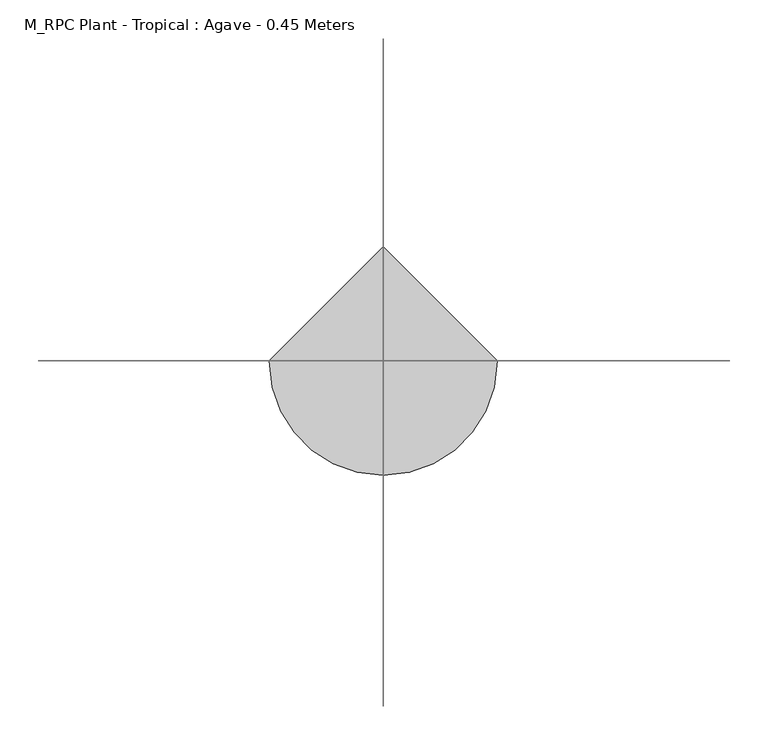
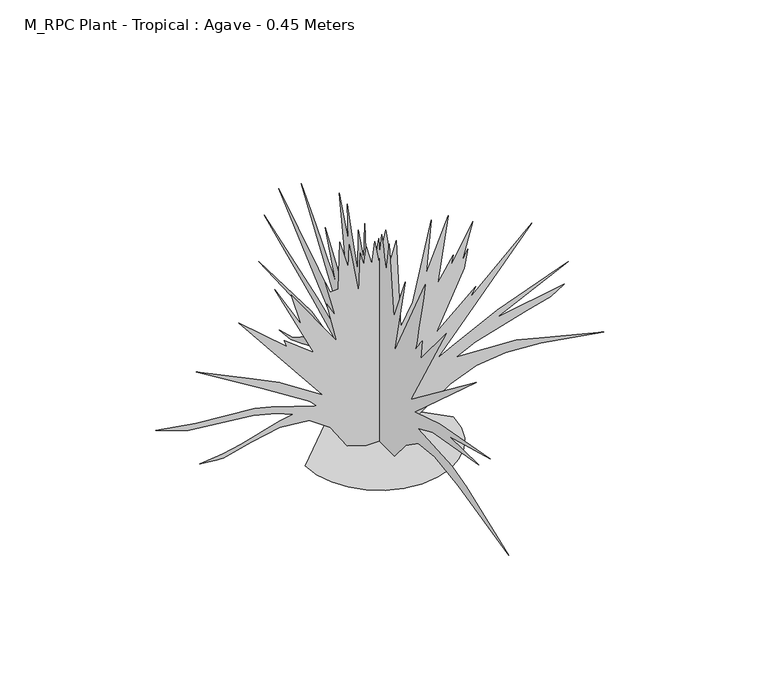
"""IFC4 building model written with IfcOpenShell, lengths in millimetres: geographic element geometry, M_RPC Plant - Tropical : Agave - 0.45 Meters."""

from ifc_helpers import new_model, si_unit, origin, place, context, project, spatial, triangles, source, transform, mapped, element, save


def m_rpc_plant_tropical_agave_0_45_meters_eb57889b(model_context):
    return source(origin(), model_context, "Body", "Tessellation", [
        triangles([(-148.1386958, 0.0, 9.3e-06), (-144.2171964, -33.9885277, 9.3e-06), (-133.048683, -65.2018023, 9.3e-06), (-115.5276685, -92.7450748, 9.3e-06), (-92.5484025, -115.7243407, 9.3e-06), (-65.0051301, -133.2453552, 9.3e-06), (-33.7918577, -144.4138686, 9.3e-06), (0.1966776, -148.335368, 9.3e-06), (34.1851976, -144.4138686, 9.3e-06), (65.3984745, -133.2453552, 9.3e-06), (92.941747, -115.7243407, 9.3e-06), (115.921013, -92.7450748, 9.3e-06), (133.4420274, -65.2018023, 9.3e-06), (144.6105409, -33.9885277, 9.3e-06), (148.5320402, 1.3e-05, 9.3e-06), (0.1966516, 148.335368, 9.3e-06), (-24.3504237, 1.1e-06, 2.5e-06), (-64.1988793, 2e-06, 12.9348607), (-97.895905, 5e-07, 64.0713026), (-140.594189, 5e-07, 94.1593235), (-198.9417449, 2.8e-06, 99.5475756), (-255.4485429, 5.9e-06, 87.7748204), (-311.5910826, 9.2e-06, 73.8080584), (-324.2335885, 9.8e-06, 74.3145591), (-359.378609, 1.11e-05, 77.950311), (-313.1035629, 8.8e-06, 82.7858171), (-277.6960585, 6.8e-06, 90.344322), (-199.7057426, 2e-06, 113.0485866), (-172.7469775, 5e-07, 117.942592), (-204.8844963, 1.2e-06, 130.9928583), (-252.5285358, 2.5e-06, 143.4918682), (-382.9561306, 7.4e-06, 157.5558808), (-447.8461741, 8.9e-06, 179.7488939), (-367.8611217, 6.2e-06, 166.4181305), (-249.0960418, 1.6e-06, 156.7231191), (-216.6905162, 6e-07, 148.7013704), (-125.4831746, -1.6e-06, 119.154591), (-138.0646922, -1.9e-06, 133.1736027), (-234.3990283, -1.3e-06, 193.9569111), (-366.6486231, -4e-07, 275.4877267), (-252.1085396, -2.1e-06, 220.5199336), (-200.6204942, -2.9e-06, 195.5036553), (-113.3644194, -3.3e-06, 138.5448591), (-281.816065, -8.5e-06, 349.4127929), (-184.8657327, -7.8e-06, 265.7927153), (-189.7134928, -8.4e-06, 280.3352324), (-131.5426794, -8.2e-06, 234.2839372), (-209.1037518, -1.44e-05, 395.4653234), (-155.7804623, -1.12e-05, 302.1502344), (-176.3827294, -1.45e-05, 372.4403117), (-85.4908937, -1.07e-05, 242.7671948), (-104.8811618, -1.49e-05, 327.6002798), (-87.9146465, -1.39e-05, 297.3027469), (-108.5169137, -1.76e-05, 374.8628019), (-97.9506527, -1.66e-05, 351.3077717), (-81.76514, -1.74e-05, 351.3277923), (-79.4313889, -2.33e-05, 450.0003668), (-62.2313759, -2.06e-05, 390.7203006), (-60.0411253, -2.35e-05, 437.880358), (-40.6511115, -1.79e-05, 330.02277), (-38.2271089, -2.29e-05, 412.4328197), (-30.9558549, -2.16e-05, 384.5578134), (-26.1083514, -2.4e-05, 422.1278312), (-15.2013409, -2.2e-05, 380.9227881), (-9.1419111, -2.5e-05, 426.9753551), (-0.6586671, -2.27e-05, 380.9227881), (12.6721065, -2.7e-05, 443.9403442), (23.5791135, -2.35e-05, 377.2877993), (34.4861967, -2.62e-05, 413.6428476), (42.9694566, -1.54e-05, 227.0126877), (67.2069761, -1.91e-05, 271.8527196), (104.0335027, -3.03e-05, 433.0253491), (93.8687435, -2.34e-05, 323.9627475), (138.4672839, -3.17e-05, 430.0728404), (116.8945182, -2.27e-05, 294.8777314), (148.4037868, -2.69e-05, 343.3552774), (143.5562902, -2.54e-05, 321.5402573), (187.1843049, -3.2e-05, 400.312811), (165.3703021, -2.65e-05, 322.7527559), (177.4890573, -2.84e-05, 345.7777677), (170.9330439, -2.58e-05, 308.0802504), (114.4707654, -1.64e-05, 190.6558953), (193.2438187, -2.4e-05, 260.9452096), (181.1248092, -2.22e-05, 240.3434511), (305.9494211, -3.46e-05, 355.4727791), (116.8945182, -1.32e-05, 136.120861), (156.175787, -1.61e-05, 155.588123), (236.8716063, -2.2e-05, 195.5036553), (378.6619886, -3.14e-05, 248.8266905), (235.6598525, -2.1e-05, 179.7488939), (371.0494809, -2.83e-05, 203.1156544), (343.871961, -2.62e-05, 186.8916447), (295.8769073, -2.33e-05, 173.2968894), (192.5770716, -1.7e-05, 143.7823665), (154.4632825, -1.42e-05, 125.2138505), (274.4393895, -1.91e-05, 119.154591), (331.2944584, -2.07e-05, 104.4295814), (450.1645283, -2.41e-05, 74.3145591), (324.0894476, -1.98e-05, 94.6895782), (253.5743659, -1.7e-05, 99.5105775), (194.5445751, -1.4e-05, 92.6238249), (142.6707883, -1.05e-05, 72.2130568), (85.3409936, -5.7e-06, 33.5950265), (32.7349455, -1.4e-06, 0.0), (0.196672, 19.7673413, 8.9e-06), (0.1966732, 47.0472873, 9.8e-06), (0.1966747, 67.3315551, 19.7666418), (0.1966772, 98.1250789, 58.1885449), (0.1966793, 130.6278551, 79.4465678), (0.1966812, 171.5303912, 83.5105639), (0.1966824, 205.2991693, 71.7218077), (0.1966844, 267.9552104, 45.114788), (0.1966857, 307.0702466, 29.8075238), (0.1966874, 347.7627846, 24.6271691), (0.1966857, 300.5702436, 38.2485284), (0.1966843, 245.8184439, 73.6468083), (0.1966827, 196.7091595, 96.1225757), (0.196681, 158.7086266, 94.9168263), (0.1966826, 185.5584048, 108.6283349), (0.1966859, 252.0827055, 120.1018443), (0.1966936, 419.0128324, 127.5108488), (0.1966855, 235.0574365, 132.4853544), (0.1966818, 162.3476305, 116.8738436), (0.1966792, 117.5043466, 94.9168263), (0.1966819, 157.4268734, 125.6566015), (0.1966862, 230.1374425, 162.6691225), (0.196696, 399.8753377, 236.7079353), (0.1966859, 214.4554237, 174.9013882), (0.1966819, 145.377618, 145.8161177), (0.1966963, 348.9752832, 323.9627475), (0.1966833, 143.900864, 195.427915), (0.1966945, 270.2027113, 382.1353231), (0.1966926, 244.8639419, 353.83527), (0.1966907, 220.4639232, 326.4102725), (0.1966889, 197.940407, 300.737748), (0.1966873, 178.2316355, 277.6927156), (0.196686, 162.2761232, 258.1477059), (0.1966851, 151.0121214, 242.9834425), (0.1966845, 145.377618, 233.0721834), (0.1966896, 187.793897, 339.7177814), (0.196686, 146.5683701, 279.2777206), (0.1966856, 142.6428648, 273.9577147), (0.1966852, 137.8938633, 268.445206), (0.1966848, 132.4583575, 262.7727143), (0.1966844, 126.4736029, 256.975212), (0.1966839, 120.0768458, 251.0802049), (0.1966835, 113.4055869, 245.1219385), (0.196683, 106.5973361, 239.1316973), (0.1966904, 138.1063594, 442.7278456), (0.1966867, 107.8090899, 361.5328016), (0.196689, 111.4448418, 435.4578315), (0.196687, 96.9023247, 386.9828107), (0.1966838, 73.8763092, 315.4802347), (0.1966864, 72.6643101, 403.9478362), (0.196684, 54.4860456, 353.0502889), (0.1966862, 50.8502891, 430.6103439), (0.1966844, 46.5152885, 378.1328058), (0.1966819, 26.6125221, 322.7527559), (0.1966839, 1.1628534, 429.3978453), (0.1966829, -1.2609561, 399.1003123), (0.1966839, -8.4154066, 443.3628722), (0.1966833, -11.7897339, 429.27536), (0.1966828, -15.0040374, 415.6178361), (0.1966823, -17.8983397, 402.817818), (0.1966818, -20.312591, 391.3078011), (0.1966815, -22.0867923, 381.5153028), (0.1966812, -23.0609175, 373.8703116), (0.196681, -23.0749678, 368.8027794), (0.1966826, -33.9820282, 439.0928567), (0.1966776, -49.7365399, 293.6677398), (0.1966787, -90.9408244, 393.0427969), (0.1966754, -52.1602928, 222.165182), (0.1966767, -160.0183758, 429.3978453), (0.1966761, -153.4961177, 397.6378289), (0.1966754, -147.1613663, 367.0353001), (0.1966749, -141.2021097, 338.7452754), (0.1966744, -135.8058548, 313.9252424), (0.196674, -131.1606078, 293.7327431), (0.1966737, -127.4541026, 279.3227215), (0.1966736, -124.8736006, 271.8527196), (0.1966736, -124.0245972, 269.8952083), (0.1966736, -125.1655977, 270.9177113), (0.1966735, -127.9646002, 274.4252189), (0.1966735, -132.0906019, 279.9202323), (0.1966735, -137.2113559, 286.9052347), (0.1966735, -142.995614, 294.8852345), (0.1966734, -149.1113653, 303.3627512), (0.1966725, -143.0521149, 262.1577082), (0.1966717, -232.7319426, 370.0152781), (0.1966708, -109.1190844, 155.5111291), (0.1966659, -335.7427697, 328.8102714), (0.1966697, -122.4498477, 136.1211063), (0.1966666, -209.7059134, 163.9943868), (0.1966597, -385.1278004, 196.2989011), (0.196665, -242.4269358, 157.9348729), (0.1966604, -345.9302656, 160.358871), (0.1966667, -186.3451482, 131.3988564), (0.1966683, -133.3568582, 108.2475896), (0.1966628, -253.3352089, 100.9760767), (0.1966602, -301.8102479, 87.6453225), (0.1966519, -448.4478453, 30.686524), (0.196661, -273.6277203, 71.7218077), (0.196665, -192.0614054, 83.6695659), (0.1966673, -135.4426048, 77.7298121), (0.1966684, -92.7000739, 48.0972868), (0.1966688, -51.7737929, 6.8e-06), (0.1966702, -18.8243404, 7.8e-06)], [[15, 16, 1], [14, 15, 1], [14, 1, 2], [13, 14, 2], [13, 2, 3], [13, 3, 4], [12, 13, 4], [11, 12, 4], [11, 4, 5], [11, 5, 6], [11, 6, 7], [11, 7, 8], [11, 8, 9], [11, 9, 10], [47, 48, 49], [97, 98, 99], [88, 89, 90], [39, 40, 41], [84, 85, 86], [71, 72, 73], [53, 54, 55], [32, 33, 34], [43, 44, 45], [24, 25, 26], [58, 59, 60], [77, 78, 79], [73, 74, 75], [60, 61, 62], [51, 52, 53], [56, 57, 58], [82, 83, 84], [79, 80, 81], [64, 65, 66], [49, 50, 51], [68, 69, 70], [75, 76, 77], [90, 91, 92], [90, 92, 93], [66, 67, 68], [82, 84, 86], [90, 93, 94], [62, 63, 64], [47, 49, 51], [39, 41, 42], [45, 46, 47], [43, 45, 47], [38, 39, 42], [38, 42, 43], [31, 32, 34], [31, 34, 35], [23, 24, 26], [56, 58, 60], [87, 88, 90], [87, 90, 94], [87, 94, 95], [37, 38, 43], [86, 87, 95], [71, 73, 75], [96, 97, 99], [96, 99, 100], [95, 96, 100], [95, 100, 101], [95, 101, 102], [53, 55, 56], [53, 56, 60], [22, 23, 26], [22, 26, 27], [22, 27, 28], [21, 22, 28], [60, 62, 64], [43, 47, 51], [30, 31, 35], [30, 35, 36], [30, 36, 37], [29, 30, 37], [86, 95, 102], [21, 28, 29], [20, 21, 29], [20, 29, 37], [19, 20, 37], [86, 102, 103], [66, 68, 70], [64, 66, 70], [60, 64, 70], [53, 60, 70], [51, 53, 70], [43, 51, 70], [77, 79, 81], [77, 81, 82], [75, 77, 82], [71, 75, 82], [70, 71, 82], [70, 82, 86], [43, 70, 86], [43, 86, 103], [43, 103, 104], [43, 104, 17], [43, 17, 18], [43, 18, 19], [43, 19, 37], [120, 121, 122], [193, 194, 195], [190, 191, 192], [126, 127, 128], [155, 156, 157], [131, 132, 133], [200, 201, 202], [113, 114, 115], [195, 196, 197], [129, 130, 131], [131, 133, 134], [170, 171, 172], [188, 189, 190], [131, 134, 135], [148, 149, 150], [139, 140, 141], [131, 135, 136], [150, 151, 152], [168, 169, 170], [172, 173, 174], [131, 136, 137], [158, 159, 160], [172, 174, 175], [131, 137, 138], [153, 154, 155], [131, 138, 139], [172, 175, 176], [160, 161, 162], [172, 176, 177], [186, 187, 188], [172, 177, 178], [112, 113, 115], [112, 115, 116], [111, 112, 116], [111, 116, 117], [160, 162, 163], [172, 178, 179], [172, 179, 180], [172, 180, 181], [139, 141, 142], [193, 195, 197], [185, 186, 188], [192, 193, 197], [192, 197, 198], [155, 157, 158], [150, 152, 153], [148, 150, 153], [139, 142, 143], [199, 200, 202], [119, 120, 122], [119, 122, 123], [118, 119, 123], [199, 202, 203], [198, 199, 203], [198, 203, 204], [184, 185, 188], [110, 111, 117], [110, 117, 118], [109, 110, 118], [160, 163, 164], [118, 123, 124], [109, 118, 124], [139, 143, 144], [125, 126, 128], [125, 128, 129], [183, 184, 188], [139, 144, 145], [153, 155, 158], [108, 109, 124], [139, 145, 146], [160, 164, 165], [158, 160, 165], [158, 165, 166], [158, 166, 167], [158, 167, 168], [158, 168, 170], [182, 183, 188], [124, 125, 129], [182, 188, 190], [181, 182, 190], [172, 181, 190], [139, 146, 147], [131, 139, 147], [131, 147, 148], [158, 170, 172], [153, 158, 172], [148, 153, 172], [198, 204, 205], [131, 148, 172], [129, 131, 172], [124, 129, 172], [124, 172, 190], [108, 124, 190], [107, 108, 190], [106, 107, 190], [105, 106, 190], [207, 105, 190], [206, 207, 190], [205, 206, 190], [198, 205, 190], [192, 198, 190]], closed=False),
    ])


if __name__ == "__main__":
    model = new_model("IFC4")
    model_context = context("Model", 3, world=origin())
    ifc_project = project(units=[si_unit("LENGTHUNIT", "METRE", prefix="MILLI")], contexts=[model_context])
    site = spatial("IfcSite", under=ifc_project)
    building = spatial("IfcBuilding", under=site)
    placement = place(None, origin())
    m_rpc_plant_tropical_agave_0_45_meters_shape = m_rpc_plant_tropical_agave_0_45_meters_eb57889b(model_context)
    element("IfcGeographicElement", 1, ObjectType="M_RPC Plant - Tropical : Agave - 0.45 Meters", at=placement, inside=building, context=model_context, shape_type="MappedRepresentation", body=[
        mapped(m_rpc_plant_tropical_agave_0_45_meters_shape, transform((0.0, 0.0, 0.0), x_axis=(1.0, 0.0, 0.0), y_axis=(0.0, 1.0, 0.0), z_axis=(0.0, 0.0, 1.0))),
    ])
    save(model, "model.ifc")

# Revit data of these elements
# Type "M_RPC Plant - Tropical : Agave - 0.45 Meters"
#   built-in parameter 1005198 = "{2, 15},{39, RPC-16-G1GJ-63FX-7K5P-N000-ST1L-LVER-AU},{1, 0},{1, 0},{2, 35},{1, 8},{5, Color},{1, 0},{1, 0},{3, 0.8},{3, 0.8},{3, 0.8},{1, 8},{7, BBoxMin},{1, 0},{1, 0},{1, 0},{1, 0},{1, 0},{1, 8},{7, BBoxMax},{1, 0},{1, 0},{1, 0},{1, 0},{1, 0},{2, 11},{9, RPCTypeId},{1, 0},{1, 0},{39, RPC-16-G1GJ-63FX-7K5P-N000-ST1L-LVER-AU},{1, 6},{14, RPCPlantHeight},{1, 0},{1, 0},{7, 1.47638},{2, 11},{7, keyword},{1, 0},{1, 0},{88, :Geometry:RPC:Agave:agave:agave americana marginata:mesqual:south western:tropical:plant},{2, 11},{8, category},{1, 0},{1, 0},{17, :Plants [General]},{2, 11},{12, LocalizedUID},{1, 0},{1, 0},{5, Agave},{2, 14},{6, Height},{1, 0},{1, 0},{7, 1.47638},{1, 2},{16, Cast Reflections},{1, 0},{1, 0},{1, 0},{1, 2},{12, Cast Shadows},{1, 0},{1, 0},{1, 1},{1, 2},{9, Lock View},{1, 0},{1, 0},{1, 0},{1, 4},{5, ViewC},{1, 0},{1, 0},{1, 0},{2, 11},{20, AdvancedUIDefinition},{1, 0},{1, 0},{0, },{2, 11},{10, AssetLibID},{1, 0},{1, 0},{36, 4D3F6E72-3F99-4203-98E9-AF80B3C7A7A4},{2, 11},{10, BaseSchema},{1, 0},{1, 0},{9, RPCSchema},{2, 11},{12, ExchangeGUID},{1, 0},{1, 0},{0, },{1, 2},{6, Hidden},{1, 0},{1, 0},{1, 0},{1, 4},{11, RPCCategory},{1, 0},{1, 0},{1, 0},{2, 11},{8, RPCImage},{1, 0},{1, 0},{0, },{1, 4},{13, SchemaVersion},{1, 0},{1, 0},{1, 4},{2, 11},{12, UIDefinition},{1, 0},{1, 0},{0, },{2, 11},{6, UIName},{1, 0},{1, 0},{39, RPC-16-G1GJ-63FX-7K5P-N000-ST1L-LVER-AU},{2, 11},{11, VersionGUID},{1, 0},{1, 0},{9, RPCSchema},{2, 11},{9, assettype},{1, 0},{1, 0},{11, RPCGeometry},{2, 11},{11, description},{1, 0},{1, 0},{0, },{2, 11},{9, localname},{1, 0},{1, 0},{3, RPC},{2, 11},{9, localtype},{1, 0},{1, 0},{3, RPC},{1, 4},{8, revision},{1, 0},{1, 0},{1, 1},{2, 11},{9, thumbnail},{1, 0},{1, 0},{0, },{1, 4},{7, version},{1, 0},{1, 0},{1, 1},{1, 2},{20, RPC_Cast Reflections},{1, 0},{1, 0},{1, 1},{1, 2},{16, RPC_Cast Shadows},{1, 0},{1, 0},{1, 1},{1, 2},{13, RPC_Lock View},{1, 0},{1, 0},{1, 0},{1, 4},{9, RPC_ViewC},{1, 0},{1, 0},{1, 0},{21, assetlibrary_base.fbx},{1, 5},"
#   built-in parameter 1005195 = "RPC-16-G1GJ-63FX-7K5P-N000-ST1L-LVER-AU"
#   Type Comments = "Agave"
#   Height = 1' - 5.71654"
#   Description = (empty or 0)
#   Default Elevation = 0
